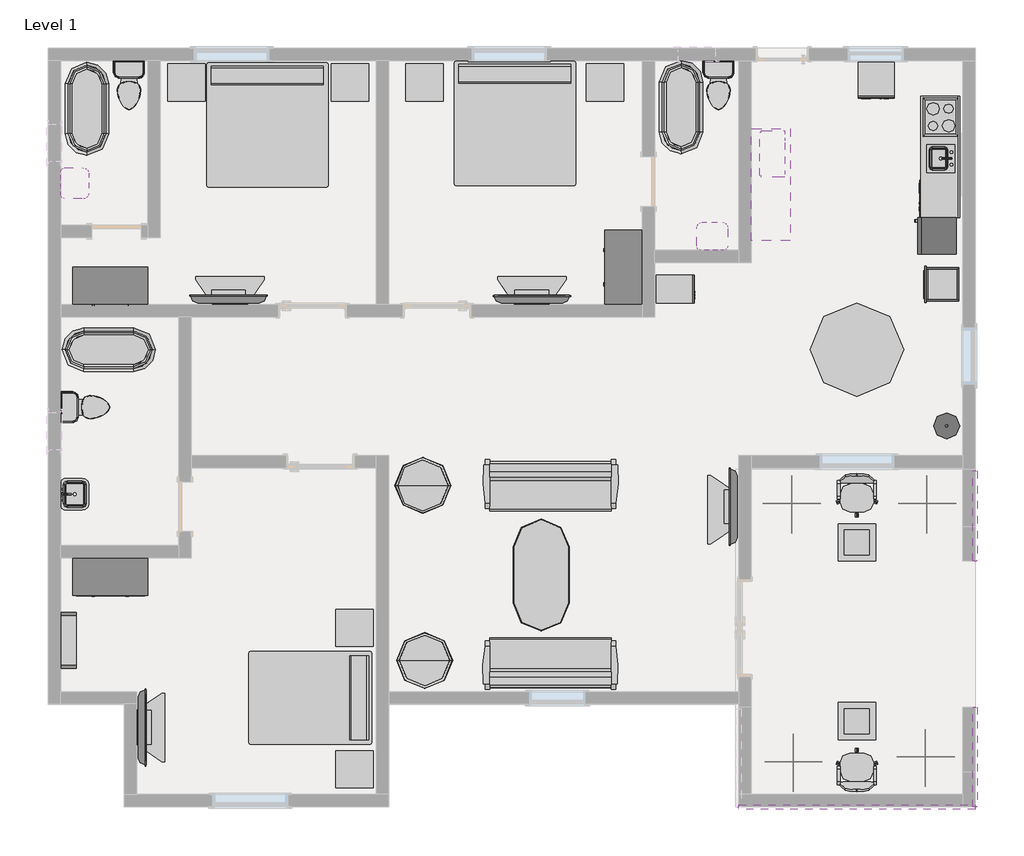
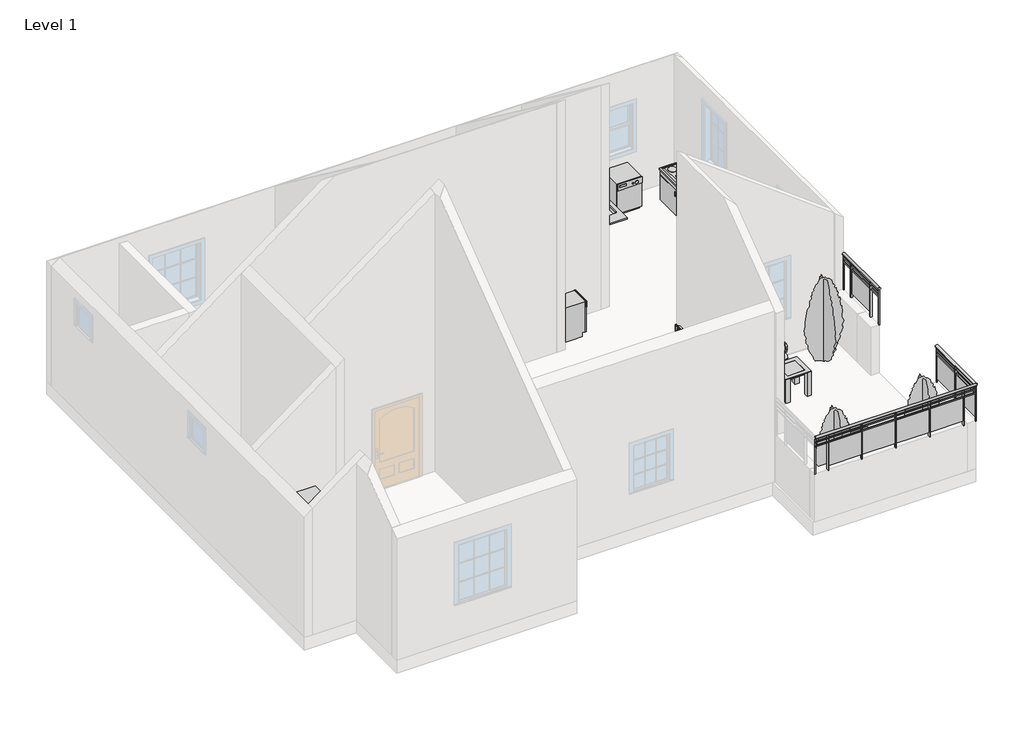
# One storey, part 2 of 2: 33 furniture elements, 11 flow terminals, 8 proxies, 4 geographic elements, 3 railings.
"""IFC4 building model written with IfcOpenShell, lengths in millimetres."""

from ifc_helpers import new_model, si_unit, point, frame, origin, place, context, project, spatial, polyline, ellipse_curve, trimmed, outline, extrude, transform, mapped, element, save
from ifc_brep_helpers import plane_surface, extruded_surface, advanced_brep
from components import proxy_7e1014cc, proxy_a6faaae8, proxy_53e5fb40, proxy_45b28599, kitchenette_medium_kitchenette_medium_844211aa, proxy_8a8d5ab2, proxy_8b8c2dc4, proxy_c523a7b7, flow_terminal_871c2e40, flow_terminal_d49f872f, flow_terminal_62a433f7, toilet_domestic_3d_toilet_domestic_3d_f7549cf7, toilet_domestic_3d_toilet_domestic_3d_183bbd19, flow_terminal_9fc66f1c, furniture_1fc5af50, furniture_e1791683, chair_executive_chair_executive_8d69e98c, furniture_c6510c7c, furniture_1447f48d, furniture_9fa109b2, furniture_417d203a, furniture_aff9b2fb, furniture_fdf74506, tv_stand_tv_stand_6ce107e5, furniture_b5c51a22, furniture_2c34a4f9, furniture_bbcc68ce, furniture_5bc9ed15, furniture_c80d6d9c, rpc_tree_conifer_chinese_juniper_7_1b9786cd

model = new_model("IFC4")

# Units and contexts
model_context = context("Model", 3, world=origin())
ifc_project = project(units=[si_unit("LENGTHUNIT", "METRE", prefix="MILLI")], contexts=[model_context])

# Site, building, storey
site = spatial("IfcSite", under=ifc_project)
building = spatial("IfcBuilding", under=site)
storey = spatial("IfcBuildingStorey", under=building, Name="Level 1", Elevation=0.0)

# Proxies
placement = place(None, origin())
proxy_shape = proxy_7e1014cc(model_context)
element("IfcBuildingElementProxy", 1, Name="18\" x 24\" x 34 1/2\"", ObjectType="18\" x 24\" x 34 1/2\"", at=placement, inside=storey, context=model_context, shape_type="MappedRepresentation", body=[
    mapped(proxy_shape, transform((-2808.5456342, 2713.390204, 0.0), x_axis=(0.0, 1.0000000000000002, 0.0), y_axis=(-1.0000000000000002, 0.0, 0.0), z_axis=(0.0, 0.0, 1.0))),
])
proxy_2_shape = proxy_a6faaae8(model_context)
element("IfcBuildingElementProxy", 2, Name="Cook Top-4 Unit2 : 22\" x 20\"", ObjectType="Cook Top-4 Unit2 : 22\" x 20\"", at=placement, inside=storey, context=model_context, shape_type="MappedRepresentation", body=[
    mapped(proxy_2_shape, transform((1268.404801, 5826.2076725, 0.0), x_axis=(0.0, -1.0, 0.0), y_axis=(1.0, 0.0, 0.0), z_axis=(0.0, 0.0, 1.0))),
])
proxy_3_shape = proxy_53e5fb40(model_context)
element("IfcBuildingElementProxy", 3, Name="Dishwasher : 23\" x 23 11/16\" x 33 1/2\"", ObjectType="Dishwasher : 23\" x 23 11/16\" x 33 1/2\"", at=placement, inside=storey, context=model_context, shape_type="MappedRepresentation", body=[
    mapped(proxy_3_shape, transform((-155.3126675, 6189.9956077, 0.0), x_axis=(1.0, 0.0, 0.0), y_axis=(0.0, 1.0, 0.0), z_axis=(0.0, 0.0, 1.0))),
])
proxy_4_shape = proxy_45b28599(model_context)
element("IfcBuildingElementProxy", 4, Name="Dishwasher : 24\" x 24\" x 34\"", ObjectType="Dishwasher : 24\" x 24\" x 34\"", at=placement, inside=storey, context=model_context, shape_type="MappedRepresentation", body=[
    mapped(proxy_4_shape, transform((976.5552362, 4875.025141, 0.0), x_axis=(0.0, -1.0, 0.0), y_axis=(1.0, 0.0, 0.0), z_axis=(0.0, 0.0, 1.0))),
])
kitchenette_medium_kitchenette_medium_shape = kitchenette_medium_kitchenette_medium_844211aa(model_context)
element("IfcBuildingElementProxy", 5, Name="Kitchenette - Medium : Kitchenette - Medium", ObjectType="Kitchenette - Medium : Kitchenette - Medium", at=placement, inside=storey, context=model_context, shape_type="MappedRepresentation", body=[
    mapped(kitchenette_medium_kitchenette_medium_shape, transform((1573.204801, 5502.0453774, 0.0), x_axis=(0.0, -1.0, 0.0), y_axis=(1.0, 0.0, 0.0), z_axis=(0.0, 0.0, 1.0))),
])
proxy_5_shape = proxy_8a8d5ab2(model_context)
element("IfcBuildingElementProxy", 6, Name="Microwave : 30\" x 16\" x 18\"", ObjectType="Microwave : 30\" x 16\" x 18\"", at=placement, inside=storey, context=model_context, shape_type="MappedRepresentation", body=[
    mapped(proxy_5_shape, transform((-1840.5757048, 4729.0147952, 914.4), x_axis=(0.0, 1.0000000000000002, 0.0), y_axis=(-1.0000000000000002, 0.0, 0.0), z_axis=(0.0, 0.0, 1.0))),
])
proxy_6_shape = proxy_8b8c2dc4(model_context)
element("IfcBuildingElementProxy", 7, Name="Oven Double-Built-in : 21 1/2\" x 39 1/4\" x 21\"", ObjectType="Oven Double-Built-in : 21 1/2\" x 39 1/4\" x 21\"", at=placement, inside=storey, context=model_context, shape_type="MappedRepresentation", body=[
    mapped(proxy_6_shape, transform((1152.7389421, 3060.5327452, 0.0), x_axis=(0.0, -1.0000000000000007, 0.0), y_axis=(1.0000000000000007, 0.0, 0.0), z_axis=(0.0, 0.0, 1.0))),
])
proxy_7_shape = proxy_c523a7b7(model_context)
element("IfcBuildingElementProxy", 8, Name="Refrigerator : 24\" x 25\" LH", ObjectType="Refrigerator : 24\" x 25\" LH", at=placement, inside=storey, context=model_context, shape_type="MappedRepresentation", body=[
    mapped(proxy_7_shape, transform((1222.7558295, 3889.4576725, 0.0), x_axis=(0.0, -1.0, 0.0), y_axis=(1.0, 0.0, 0.0), z_axis=(0.0, 0.0, 1.0))),
])

# Flow terminals
flow_terminal_shape = flow_terminal_871c2e40(model_context)
element("IfcFlowTerminal", 9, ObjectType="Sink Kitchen-Island : 18\" x 18\"", at=placement, inside=storey, context=model_context, shape_type="MappedRepresentation", body=[
    mapped(flow_terminal_shape, transform((1266.0593999, 5168.7969131, -14.4), x_axis=(0.0, -1.0, 0.0), y_axis=(1.0, 0.0, 0.0), z_axis=(0.0, 0.0, 1.0))),
])
flow_terminal_2_shape = flow_terminal_d49f872f(model_context)
element("IfcFlowTerminal", 10, ObjectType="Sink Vanity-Round : 19\" x 19\"", at=placement, inside=storey, context=model_context, shape_type="MappedRepresentation", body=[
    mapped(flow_terminal_2_shape, transform((1277.3399031, 880.9594131, 609.6), x_axis=(0.0, -1.0000000000000004, 0.0), y_axis=(1.0000000000000004, 0.0, 0.0), z_axis=(0.0, 0.0, 1.0))),
])
flow_terminal_3_shape = flow_terminal_62a433f7(model_context)
element("IfcFlowTerminal", 11, ObjectType="Sink Vanity-Square : 20\" x 18\"", at=placement, inside=storey, context=model_context, shape_type="MappedRepresentation", body=[
    mapped(flow_terminal_3_shape, transform((-12927.8497979, -348.9815681, 0.0), x_axis=(0.0, 1.0000000000000002, 0.0), y_axis=(-1.0000000000000002, 0.0, 0.0), z_axis=(0.0, 0.0, 1.0))),
])
element("IfcFlowTerminal", 12, ObjectType="Sink Vanity-Square : 20\" x 18\"", at=placement, inside=storey, context=model_context, shape_type="MappedRepresentation", body=[
    mapped(flow_terminal_3_shape, transform((-12927.8497979, 4731.0184319, 914.4), x_axis=(0.0, 1.0000000000000002, 0.0), y_axis=(-1.0000000000000002, 0.0, 0.0), z_axis=(0.0, 0.0, 1.0))),
])
element("IfcFlowTerminal", 13, ObjectType="Sink Vanity-Square : 20\" x 18\"", at=placement, inside=storey, context=model_context, shape_type="MappedRepresentation", body=[
    mapped(flow_terminal_3_shape, transform((-2449.7059584, 3834.6530736, 914.4), x_axis=(-1.0, 0.0, 0.0), y_axis=(0.0, -1.0, 0.0), z_axis=(0.0, 0.0, 1.0))),
])
toilet_domestic_3d_toilet_domestic_3d_shape = toilet_domestic_3d_toilet_domestic_3d_f7549cf7(model_context)
toilet_domestic_3d_toilet_domestic_3d_2_shape = toilet_domestic_3d_toilet_domestic_3d_183bbd19(model_context)
element("IfcFlowTerminal", 14, ObjectType="Toilet-Domestic-3D : Toilet-Domestic-3D", at=placement, inside=storey, context=model_context, shape_type="MappedRepresentation", body=[
    mapped(toilet_domestic_3d_toilet_domestic_3d_shape, transform((-12613.2991716, 1089.1076725, 0.0), x_axis=(0.0, 1.0000000000000002, 0.0), y_axis=(-1.0000000000000002, 0.0, 0.0), z_axis=(0.0, 0.0, 1.0))),
    mapped(toilet_domestic_3d_toilet_domestic_3d_2_shape, transform((-12613.2991716, 1089.1076725, 0.0), x_axis=(0.0, 1.0000000000000002, 0.0), y_axis=(-1.0000000000000002, 0.0, 0.0), z_axis=(0.0, 0.0, 1.0))),
])
element("IfcFlowTerminal", 15, ObjectType="Toilet-Domestic-3D : Toilet-Domestic-3D", at=placement, inside=storey, context=model_context, shape_type="MappedRepresentation", body=[
    mapped(toilet_domestic_3d_toilet_domestic_3d_shape, transform((-11990.395199, 6258.6116451, 0.0), x_axis=(1.0, 0.0, 0.0), y_axis=(0.0, 1.0, 0.0), z_axis=(0.0, 0.0, 1.0))),
    mapped(toilet_domestic_3d_toilet_domestic_3d_2_shape, transform((-11990.395199, 6258.6116451, 0.0), x_axis=(1.0, 0.0, 0.0), y_axis=(0.0, 1.0, 0.0), z_axis=(0.0, 0.0, 1.0))),
])
element("IfcFlowTerminal", 16, ObjectType="Toilet-Domestic-3D : Toilet-Domestic-3D", at=placement, inside=storey, context=model_context, shape_type="MappedRepresentation", body=[
    mapped(toilet_domestic_3d_toilet_domestic_3d_shape, transform((-2363.795199, 6258.6116451, 0.0), x_axis=(1.0, 0.0, 0.0), y_axis=(0.0, 1.0, 0.0), z_axis=(0.0, 0.0, 1.0))),
    mapped(toilet_domestic_3d_toilet_domestic_3d_2_shape, transform((-2363.795199, 6258.6116451, 0.0), x_axis=(1.0, 0.0, 0.0), y_axis=(0.0, 1.0, 0.0), z_axis=(0.0, 0.0, 1.0))),
])
flow_terminal_4_shape = flow_terminal_9fc66f1c(model_context)
element("IfcFlowTerminal", 17, ObjectType="Tub-Free Standing-3D : 30\" x 60\"", at=placement, inside=storey, context=model_context, shape_type="MappedRepresentation", body=[
    mapped(flow_terminal_4_shape, transform((-12320.595199, 2028.9076725, 0.0), x_axis=(0.0, 1.0000000000000009, 0.0), y_axis=(-1.0000000000000009, 0.0, 0.0), z_axis=(0.0, 0.0, 1.0))),
])
element("IfcFlowTerminal", 18, ObjectType="Tub-Free Standing-3D : 30\" x 60\"", at=placement, inside=storey, context=model_context, shape_type="MappedRepresentation", body=[
    mapped(flow_terminal_4_shape, transform((-12676.195199, 5965.9076725, 0.0), x_axis=(1.0, 0.0, 0.0), y_axis=(0.0, 1.0, 0.0), z_axis=(0.0, 0.0, 1.0))),
])
element("IfcFlowTerminal", 19, ObjectType="Tub-Free Standing-3D : 30\" x 60\"", at=placement, inside=storey, context=model_context, shape_type="MappedRepresentation", body=[
    mapped(flow_terminal_4_shape, transform((-2973.395199, 5991.3076725, 0.0), x_axis=(1.0, 0.0, 0.0), y_axis=(0.0, 1.0, 0.0), z_axis=(0.0, 0.0, 1.0))),
])

# Furniture
furniture_shape = furniture_1fc5af50(model_context)
element("IfcFurniture", 20, ObjectType="Bed-Standard.0001 : King 78\" x 80\"", at=placement, inside=storey, context=model_context, shape_type="MappedRepresentation", body=[
    mapped(furniture_shape, transform((-10001.2837236, 5744.8027545, 0.0), x_axis=(1.0, 0.0, 0.0), y_axis=(0.0, 1.0, 0.0), z_axis=(0.0, 0.0, 1.0))),
])
element("IfcFurniture", 21, ObjectType="Bed-Standard.0001 : King 78\" x 80\"", at=placement, inside=storey, context=model_context, shape_type="MappedRepresentation", body=[
    mapped(furniture_shape, transform((-5958.5510914, 5770.2027545, 0.0), x_axis=(1.0000000000000002, 0.0, 0.0), y_axis=(0.0, 1.0000000000000002, 0.0), z_axis=(0.0, 0.0, 1.0))),
])
furniture_2_shape = furniture_e1791683(model_context)
element("IfcFurniture", 22, ObjectType="Bed-Standard.0001 : Queen 60\" x 79\"", at=placement, inside=storey, context=model_context, shape_type="MappedRepresentation", body=[
    mapped(furniture_2_shape, transform((-8985.700117, -3389.2038029, 0.0), x_axis=(0.0, -1.0000000000000007, 0.0), y_axis=(1.0000000000000007, 0.0, 0.0), z_axis=(0.0, 0.0, 1.0))),
])
chair_executive_chair_executive_shape = chair_executive_chair_executive_8d69e98c(model_context)
element("IfcFurniture", 23, ObjectType="Chair-Executive : Chair-Executive", at=placement, inside=storey, context=model_context, shape_type="MappedRepresentation", body=[
    mapped(chair_executive_chair_executive_shape, transform((37.7956207, -339.7464259, 0.0), x_axis=(-1.0000000000000002, 0.0, 0.0), y_axis=(0.0, -1.0000000000000002, 0.0), z_axis=(0.0, 0.0, 1.0))),
])
element("IfcFurniture", 24, ObjectType="Chair-Executive : Chair-Executive", at=placement, inside=storey, context=model_context, shape_type="MappedRepresentation", body=[
    mapped(chair_executive_chair_executive_shape, transform((-244.1860187, -4848.0382291, 0.0), x_axis=(1.0000000000000002, 0.0, 0.0), y_axis=(0.0, 1.0000000000000002, 0.0), z_axis=(0.0, 0.0, 1.0))),
])
furniture_3_shape = furniture_c6510c7c(model_context)
element("IfcFurniture", 25, ObjectType="Counter Top w Sink Hole : 24\" Depth", at=placement, inside=storey, context=model_context, shape_type="MappedRepresentation", body=[
    mapped(furniture_3_shape, transform((1573.204801, 4968.6453774, -14.4), x_axis=(0.0, -1.0, 0.0), y_axis=(1.0, 0.0, 0.0), z_axis=(0.0, 0.0, 1.0))),
])
furniture_4_shape = furniture_1447f48d(model_context)
element("IfcFurniture", 26, ObjectType="Counter Top w Sink Hole : 24\" Depth", at=placement, inside=storey, context=model_context, shape_type="MappedRepresentation", body=[
    mapped(furniture_4_shape, transform((-1830.395199, 5007.3699676, 914.4), x_axis=(0.0, 1.0000000000000002, 0.0), y_axis=(-1.0000000000000002, 0.0, 0.0), z_axis=(0.0, 0.0, 1.0))),
])
furniture_5_shape = furniture_9fa109b2(model_context)
element("IfcFurniture", 27, ObjectType="Dresser : 48\" x 72\" x 24\"", at=placement, inside=storey, context=model_context, shape_type="MappedRepresentation", body=[
    mapped(furniture_5_shape, transform((-12026.0019391, 3433.4706266, 0.0), x_axis=(1.0, 0.0, 0.0), y_axis=(0.0, 1.0, 0.0), z_axis=(0.0, 0.0, 1.0))),
])
element("IfcFurniture", 28, ObjectType="Dresser : 48\" x 72\" x 24\"", at=placement, inside=storey, context=model_context, shape_type="MappedRepresentation", body=[
    mapped(furniture_5_shape, transform((-12026.0019391, -1316.3293734, 0.0), x_axis=(1.0, 0.0, 0.0), y_axis=(0.0, 1.0, 0.0), z_axis=(0.0, 0.0, 1.0))),
])
element("IfcFurniture", 29, ObjectType="Dresser : 48\" x 72\" x 24\"", at=placement, inside=storey, context=model_context, shape_type="MappedRepresentation", body=[
    mapped(furniture_5_shape, transform((-3550.0322449, 3105.9144127, 0.0), x_axis=(0.0, -1.0000000000000004, 0.0), y_axis=(1.0000000000000004, 0.0, 0.0), z_axis=(0.0, 0.0, 1.0))),
])
furniture_6_shape = furniture_417d203a(model_context)
element("IfcFurniture", 30, ObjectType="Shelving : 36\" x 10\" x 72\"", at=placement, inside=storey, context=model_context, shape_type="MappedRepresentation", body=[
    mapped(furniture_6_shape, transform((-13285.795199, -2720.8923275, 0.0), x_axis=(0.0, 1.0, 0.0), y_axis=(-1.0, 0.0, 0.0), z_axis=(0.0, 0.0, 1.0))),
])
furniture_7_shape = furniture_aff9b2fb(model_context)
element("IfcFurniture", 31, ObjectType="Sofa-Pensi : 84\"", at=placement, inside=storey, context=model_context, shape_type="MappedRepresentation", body=[
    mapped(furniture_7_shape, transform((-5385.601449, -464.3521636, 0.0), x_axis=(1.0000000000000009, 0.0, 0.0), y_axis=(0.0, 1.0000000000000009, 0.0), z_axis=(0.0, 0.0, 1.0))),
])
element("IfcFurniture", 32, ObjectType="Sofa-Pensi : 84\"", at=placement, inside=storey, context=model_context, shape_type="MappedRepresentation", body=[
    mapped(furniture_7_shape, transform((-4828.388949, -2824.7824914, 0.0), x_axis=(-1.0, 0.0, 0.0), y_axis=(0.0, -1.0, 0.0), z_axis=(0.0, 0.0, 1.0))),
])
furniture_8_shape = furniture_fdf74506(model_context)
element("IfcFurniture", 33, ObjectType="TV - Flat Screen : 50\"", at=placement, inside=storey, context=model_context, shape_type="MappedRepresentation", body=[
    mapped(furniture_8_shape, transform((-10368.7397131, 2850.4920708, 914.4), x_axis=(-1.0, 0.0, 0.0), y_axis=(0.0, -1.0, 0.0), z_axis=(0.0, 0.0, 1.0))),
])
element("IfcFurniture", 34, ObjectType="TV - Flat Screen : 50\"", at=placement, inside=storey, context=model_context, shape_type="MappedRepresentation", body=[
    mapped(furniture_8_shape, transform((-5415.7397131, 2847.8196508, 914.4), x_axis=(-1.0, 0.0, 0.0), y_axis=(0.0, -1.0, 0.0), z_axis=(0.0, 0.0, 1.0))),
])
element("IfcFurniture", 35, ObjectType="TV - Flat Screen : 50\"", at=placement, inside=storey, context=model_context, shape_type="MappedRepresentation", body=[
    mapped(furniture_8_shape, transform((-11779.4565753, -4139.3478134, 914.4), x_axis=(0.0, 1.0000000000000002, 0.0), y_axis=(-1.0000000000000002, 0.0, 0.0), z_axis=(0.0, 0.0, 1.0))),
])
element("IfcFurniture", 36, ObjectType="TV - Flat Screen : 50\"", at=placement, inside=storey, context=model_context, shape_type="MappedRepresentation", body=[
    mapped(furniture_8_shape, transform((-2117.5338226, -540.4368416, 914.4), x_axis=(0.0, -1.0000000000000002, 0.0), y_axis=(1.0000000000000002, 0.0, 0.0), z_axis=(0.0, 0.0, 1.0))),
])
tv_stand_tv_stand_shape = tv_stand_tv_stand_6ce107e5(model_context)
element("IfcFurniture", 37, ObjectType="TV Stand : TV Stand", at=placement, inside=storey, context=model_context, shape_type="MappedRepresentation", body=[
    mapped(tv_stand_tv_stand_shape, transform((-11863.395199, -4268.4803296, 0.0), x_axis=(0.0, 1.0, 0.0), y_axis=(-1.0, 0.0, 0.0), z_axis=(0.0, 0.0, 1.0))),
])
element("IfcFurniture", 38, ObjectType="TV Stand : TV Stand", at=placement, inside=storey, context=model_context, shape_type="MappedRepresentation", body=[
    mapped(tv_stand_tv_stand_shape, transform((-10214.2071969, 2765.5076725, 0.0), x_axis=(-1.0000000000000002, 0.0, 0.0), y_axis=(0.0, -1.0000000000000002, 0.0), z_axis=(0.0, 0.0, 1.0))),
])
element("IfcFurniture", 39, ObjectType="TV Stand : TV Stand", at=placement, inside=storey, context=model_context, shape_type="MappedRepresentation", body=[
    mapped(tv_stand_tv_stand_shape, transform((-5286.6071969, 2765.5076725, 0.0), x_axis=(-1.0, 0.0, 0.0), y_axis=(0.0, -1.0, 0.0), z_axis=(0.0, 0.0, 1.0))),
])
element("IfcFurniture", 40, ObjectType="TV Stand : TV Stand", at=placement, inside=storey, context=model_context, shape_type="MappedRepresentation", body=[
    mapped(tv_stand_tv_stand_shape, transform((-2084.395199, -462.1043254, 0.0), x_axis=(0.0, -1.0, 0.0), y_axis=(1.0, 0.0, 0.0), z_axis=(0.0, 0.0, 1.0))),
])
furniture_9_shape = furniture_b5c51a22(model_context)
element("IfcFurniture", 41, ObjectType="Table-Coffee : 24\" x 24\" x 24\"", at=placement, inside=storey, context=model_context, shape_type="MappedRepresentation", body=[
    mapped(furniture_9_shape, transform((-121.4609657, -4136.9034053, 0.0), x_axis=(1.0, 0.0, 0.0), y_axis=(0.0, 1.0, 0.0), z_axis=(0.0, 0.0, 1.0))),
])
element("IfcFurniture", 42, ObjectType="Table-Coffee : 24\" x 24\" x 24\"", at=placement, inside=storey, context=model_context, shape_type="MappedRepresentation", body=[
    mapped(furniture_9_shape, transform((-121.4609657, -1215.9034053, 0.0), x_axis=(1.0, 0.0, 0.0), y_axis=(0.0, 1.0, 0.0), z_axis=(0.0, 0.0, 1.0))),
])
furniture_10_shape = furniture_2c34a4f9(model_context)
element("IfcFurniture", 43, ObjectType="Table-Dining Oval : 36\" x 72\"", at=placement, inside=storey, context=model_context, shape_type="MappedRepresentation", body=[
    mapped(furniture_10_shape, transform((-5617.4935596, -1252.2726554, 0.0), x_axis=(0.0, 1.0000000000000002, 0.0), y_axis=(-1.0000000000000002, 0.0, 0.0), z_axis=(0.0, 0.0, 1.0))),
])
furniture_11_shape = furniture_bbcc68ce(model_context)
element("IfcFurniture", 44, ObjectType="Table-Dining Round w Chairs : 60\" Diameter", at=placement, inside=storey, context=model_context, shape_type="MappedRepresentation", body=[
    mapped(furniture_11_shape, transform((-206.8771662, 2213.786361, 0.0), x_axis=(1.0, 0.0, 0.0), y_axis=(0.0, 1.0, 0.0), z_axis=(0.0, 0.0, 1.0))),
])
furniture_12_shape = furniture_5bc9ed15(model_context)
element("IfcFurniture", 45, ObjectType="Table-Night Stand : 24\" x 24\" x 30\"", at=placement, inside=storey, context=model_context, shape_type="MappedRepresentation", body=[
    mapped(furniture_12_shape, transform((-8692.1288293, 6092.9076725, 0.0), x_axis=(1.0, 0.0, 0.0), y_axis=(0.0, 1.0, 0.0), z_axis=(0.0, 0.0, 1.0))),
])
element("IfcFurniture", 46, ObjectType="Table-Night Stand : 24\" x 24\" x 30\"", at=placement, inside=storey, context=model_context, shape_type="MappedRepresentation", body=[
    mapped(furniture_12_shape, transform((-11359.1288293, 6092.9076725, 0.0), x_axis=(1.0, 0.0, 0.0), y_axis=(0.0, 1.0, 0.0), z_axis=(0.0, 0.0, 1.0))),
])
element("IfcFurniture", 47, ObjectType="Table-Night Stand : 24\" x 24\" x 30\"", at=placement, inside=storey, context=model_context, shape_type="MappedRepresentation", body=[
    mapped(furniture_12_shape, transform((-7472.9288293, 6092.9076725, 0.0), x_axis=(1.0, 0.0, 0.0), y_axis=(0.0, 1.0, 0.0), z_axis=(0.0, 0.0, 1.0))),
])
element("IfcFurniture", 48, ObjectType="Table-Night Stand : 24\" x 24\" x 30\"", at=placement, inside=storey, context=model_context, shape_type="MappedRepresentation", body=[
    mapped(furniture_12_shape, transform((-4526.5288293, 6092.9076725, 0.0), x_axis=(1.0, 0.0, 0.0), y_axis=(0.0, 1.0, 0.0), z_axis=(0.0, 0.0, 1.0))),
])
element("IfcFurniture", 49, ObjectType="Table-Night Stand : 24\" x 24\" x 30\"", at=placement, inside=storey, context=model_context, shape_type="MappedRepresentation", body=[
    mapped(furniture_12_shape, transform((-8615.9288293, -2822.4923275, 0.0), x_axis=(1.0, 0.0, 0.0), y_axis=(0.0, 1.0, 0.0), z_axis=(0.0, 0.0, 1.0))),
])
element("IfcFurniture", 50, ObjectType="Table-Night Stand : 24\" x 24\" x 30\"", at=placement, inside=storey, context=model_context, shape_type="MappedRepresentation", body=[
    mapped(furniture_12_shape, transform((-8615.9288293, -5133.8923275, 0.0), x_axis=(1.0, 0.0, 0.0), y_axis=(0.0, 1.0, 0.0), z_axis=(0.0, 0.0, 1.0))),
])
furniture_13_shape = furniture_c80d6d9c(model_context)
element("IfcFurniture", 51, ObjectType="Table-Round : 36\" Diameter", at=placement, inside=storey, context=model_context, shape_type="MappedRepresentation", body=[
    mapped(furniture_13_shape, transform((-7164.395199, -3051.0923275, 0.0), x_axis=(1.0, 0.0, 0.0), y_axis=(0.0, 1.0, 0.0), z_axis=(0.0, 0.0, 1.0))),
])
element("IfcFurniture", 52, ObjectType="Table-Round : 36\" Diameter", at=placement, inside=storey, context=model_context, shape_type="MappedRepresentation", body=[
    mapped(furniture_13_shape, transform((-7189.795199, -187.2423275, 0.0), x_axis=(1.0, 0.0, 0.0), y_axis=(0.0, 1.0, 0.0), z_axis=(0.0, 0.0, 1.0))),
])

# Geographic elements
rpc_tree_conifer_chinese_juniper_7_shape = rpc_tree_conifer_chinese_juniper_7_1b9786cd(model_context)
element("IfcGeographicElement", 53, ObjectType="RPC Tree - Conifer : Chinese Juniper - 7'", at=placement, inside=storey, context=model_context, shape_type="MappedRepresentation", body=[
    mapped(rpc_tree_conifer_chinese_juniper_7_shape, transform((-1144.7918701, -4702.0923275, 0.0), x_axis=(1.0, 0.0, 0.0), y_axis=(0.0, 1.0, 0.0), z_axis=(0.0, 0.0, 1.0))),
])
element("IfcGeographicElement", 54, ObjectType="RPC Tree - Conifer : Chinese Juniper - 7'", at=placement, inside=storey, context=model_context, shape_type="MappedRepresentation", body=[
    mapped(rpc_tree_conifer_chinese_juniper_7_shape, transform((1014.2081299, -4625.8923275, 0.0), x_axis=(1.0, 0.0, 0.0), y_axis=(0.0, 1.0, 0.0), z_axis=(0.0, 0.0, 1.0))),
])
element("IfcGeographicElement", 55, ObjectType="RPC Tree - Conifer : Chinese Juniper - 7'", at=placement, inside=storey, context=model_context, shape_type="MappedRepresentation", body=[
    mapped(rpc_tree_conifer_chinese_juniper_7_shape, transform((1039.6081299, -485.6923275, 0.0), x_axis=(1.0, 0.0, 0.0), y_axis=(0.0, 1.0, 0.0), z_axis=(0.0, 0.0, 1.0))),
])
element("IfcGeographicElement", 56, ObjectType="RPC Tree - Conifer : Chinese Juniper - 7'", at=placement, inside=storey, context=model_context, shape_type="MappedRepresentation", body=[
    mapped(rpc_tree_conifer_chinese_juniper_7_shape, transform((-1170.1918701, -485.6923275, 0.0), x_axis=(1.0, 0.0, 0.0), y_axis=(0.0, 1.0, 0.0), z_axis=(0.0, 0.0, 1.0))),
])

# Railings
element("IfcRailing", 57, ObjectType="Glass Panel - Bottom Fill", at=placement, inside=storey, context=model_context, shape_type="SolidModel", body=[
    advanced_brep(
    [(-2033.595199, -5406.9423275, 2133.6), (-2033.595199, -5483.1423275, 2133.6), (1827.204801, -5406.9423275, 2133.6), (1827.204801, -5483.1423275, 2133.6)],
    [
        (0, 1, ellipse_curve(frame((-2033.595199, -5445.0423275, 2133.6), z_axis=(-1.0, 0.0, 0.0), x_axis=(0.0, -1.0, 0.0)), 38.1, 28.575)),
        (1, 0, ellipse_curve(frame((-2033.595199, -5445.0423275, 2133.6), z_axis=(-1.0, 0.0, 0.0), x_axis=(0.0, -1.0, 0.0)), 38.1, 28.575)),
        (2, 3, ellipse_curve(frame((1827.204801, -5445.0423275, 2133.6), z_axis=(1.0, 0.0, 0.0), x_axis=(0.0, -1.0, 0.0)), 38.1, 28.575)),
        (3, 2, ellipse_curve(frame((1827.204801, -5445.0423275, 2133.6), z_axis=(1.0, 0.0, 0.0), x_axis=(0.0, -1.0, 0.0)), 38.1, 28.575)),
        (0, 2),
        (3, 1),
    ],
    [
        plane_surface(frame((-2033.595199, -5445.0423275, 2133.6), z_axis=(-1.0, 0.0, 0.0), x_axis=(0.0, 1.0, 0.0))),
        plane_surface(frame((1827.204801, -5445.0423275, 2133.6), z_axis=(1.0, 0.0, 0.0), x_axis=(0.0, 1.0, 0.0))),
        extruded_surface(trimmed(ellipse_curve(frame((1827.204801, -5445.0423275, 2133.6), z_axis=(-1.0, 0.0, 0.0), x_axis=(0.0, -1.0, 0.0)), 38.1, 28.575), [point((1827.204801, -5406.9423275, 2133.6))], [point((1827.204801, -5483.1423275, 2133.6))], True, "CARTESIAN"), (-3860.8, 0.0, 0.0), 3860.8),
        extruded_surface(trimmed(ellipse_curve(frame((1827.204801, -5445.0423275, 2133.6), z_axis=(-1.0, 0.0, 0.0), x_axis=(0.0, -1.0, 0.0)), 38.1, 28.575), [point((1827.204801, -5483.1423275, 2133.6))], [point((1827.204801, -5406.9423275, 2133.6))], True, "CARTESIAN"), (-3860.8, 0.0, 0.0), 3860.8),
    ],
    [
        (0, [[1, 2]]),
        (1, [[3, 4]]),
        (2, [[-1, 5, -4, 6]]),
        (3, [[-2, -6, -3, -5]]),
    ],
),
    extrude(outline(polyline([(-2033.595199, -5457.7423275), (-2033.595199, -5432.3423275), (1827.204801, -5432.3423275), (1827.204801, -5457.7423275), (-2033.595199, -5457.7423275)])), frame((0.0, 0.0, 2019.3), z_axis=(0.0, 0.0, 1.0), x_axis=(1.0, 0.0, 0.0)), (0.0, 0.0, 1.0), 25.4),
    extrude(outline(polyline([(-2033.595199, -5457.7423275), (-2033.595199, -5432.3423275), (1827.204801, -5432.3423275), (1827.204801, -5457.7423275), (-2033.595199, -5457.7423275)])), frame((0.0, 0.0, 1917.7), z_axis=(0.0, 0.0, 1.0), x_axis=(1.0, 0.0, 0.0)), (0.0, 0.0, 1.0), 25.4),
    extrude(outline(polyline([(1516.054801, -5470.4423275), (1516.054801, -5419.6423275), (1528.754801, -5419.6423275), (1528.754801, -5470.4423275), (1516.054801, -5470.4423275)])), frame((0.0, 0.0, 1219.2), z_axis=(0.0, 0.0, 1.0), x_axis=(1.0, 0.0, 0.0)), (0.0, 0.0, 1.0), 885.6788223),
    extrude(outline(polyline([(709.604801, -5438.5071705), (1522.404801, -5438.5071705), (1522.404801, -5444.8571705), (709.604801, -5444.8571705), (709.604801, -5438.5071705)])), frame((0.0, 0.0, 1320.8), z_axis=(0.0, 0.0, 1.0), x_axis=(1.0, 0.0, 0.0)), (0.0, 0.0, 1.0), 596.9),
    extrude(outline(polyline([(703.254801, -5470.4423275), (703.254801, -5419.6423275), (715.954801, -5419.6423275), (715.954801, -5470.4423275), (703.254801, -5470.4423275)])), frame((0.0, 0.0, 1219.2), z_axis=(0.0, 0.0, 1.0), x_axis=(1.0, 0.0, 0.0)), (0.0, 0.0, 1.0), 885.6788223),
    extrude(outline(polyline([(-103.195199, -5438.5071705), (709.604801, -5438.5071705), (709.604801, -5444.8571705), (-103.195199, -5444.8571705), (-103.195199, -5438.5071705)])), frame((0.0, 0.0, 1320.8), z_axis=(0.0, 0.0, 1.0), x_axis=(1.0, 0.0, 0.0)), (0.0, 0.0, 1.0), 596.9),
    extrude(outline(polyline([(-109.545199, -5470.4423275), (-109.545199, -5419.6423275), (-96.845199, -5419.6423275), (-96.845199, -5470.4423275), (-109.545199, -5470.4423275)])), frame((0.0, 0.0, 1219.2), z_axis=(0.0, 0.0, 1.0), x_axis=(1.0, 0.0, 0.0)), (0.0, 0.0, 1.0), 885.6788223),
    extrude(outline(polyline([(-915.995199, -5438.5071705), (-103.195199, -5438.5071705), (-103.195199, -5444.8571705), (-915.995199, -5444.8571705), (-915.995199, -5438.5071705)])), frame((0.0, 0.0, 1320.8), z_axis=(0.0, 0.0, 1.0), x_axis=(1.0, 0.0, 0.0)), (0.0, 0.0, 1.0), 596.9),
    extrude(outline(polyline([(-922.345199, -5470.4423275), (-922.345199, -5419.6423275), (-909.645199, -5419.6423275), (-909.645199, -5470.4423275), (-922.345199, -5470.4423275)])), frame((0.0, 0.0, 1219.2), z_axis=(0.0, 0.0, 1.0), x_axis=(1.0, 0.0, 0.0)), (0.0, 0.0, 1.0), 885.6788223),
    extrude(outline(polyline([(-1728.795199, -5438.5071705), (-915.995199, -5438.5071705), (-915.995199, -5444.8571705), (-1728.795199, -5444.8571705), (-1728.795199, -5438.5071705)])), frame((0.0, 0.0, 1320.8), z_axis=(0.0, 0.0, 1.0), x_axis=(1.0, 0.0, 0.0)), (0.0, 0.0, 1.0), 596.9),
    extrude(outline(polyline([(-1735.145199, -5470.4423275), (-1735.145199, -5419.6423275), (-1722.445199, -5419.6423275), (-1722.445199, -5470.4423275), (-1735.145199, -5470.4423275)])), frame((0.0, 0.0, 1219.2), z_axis=(0.0, 0.0, 1.0), x_axis=(1.0, 0.0, 0.0)), (0.0, 0.0, 1.0), 885.6788223),
    extrude(outline(polyline([(1814.504801, -5454.5673275), (1814.504801, -5435.5173275), (1833.554801, -5435.5173275), (1833.554801, -5454.5673275), (1814.504801, -5454.5673275)])), frame((0.0, 0.0, 1219.2), z_axis=(0.0, 0.0, 1.0), x_axis=(1.0, 0.0, 0.0)), (0.0, 0.0, 1.0), 885.6788223),
    extrude(outline(polyline([(-2039.945199, -5454.5673275), (-2039.945199, -5435.5173275), (-2020.895199, -5435.5173275), (-2020.895199, -5454.5673275), (-2039.945199, -5454.5673275)])), frame((0.0, 0.0, 1219.2), z_axis=(0.0, 0.0, 1.0), x_axis=(1.0, 0.0, 0.0)), (0.0, 0.0, 1.0), 885.6788223),
])
element("IfcRailing", 58, ObjectType="Glass Panel - Bottom Fill", at=placement, inside=storey, context=model_context, shape_type="SolidModel", body=[
    advanced_brep(
    [(1789.104801, -5438.6923275, 2133.6), (1865.304801, -5438.6923275, 2133.6), (1789.104801, -3813.0923275, 2133.6), (1865.304801, -3813.0923275, 2133.6)],
    [
        (0, 1, ellipse_curve(frame((1827.204801, -5438.6923275, 2133.6), z_axis=(0.0, -1.0, 0.0), x_axis=(1.0, 0.0, 0.0)), 38.1, 28.575)),
        (1, 0, ellipse_curve(frame((1827.204801, -5438.6923275, 2133.6), z_axis=(0.0, -1.0, 0.0), x_axis=(1.0, 0.0, 0.0)), 38.1, 28.575)),
        (2, 3, ellipse_curve(frame((1827.204801, -3813.0923275, 2133.6), z_axis=(0.0, 1.0, 0.0), x_axis=(1.0, 0.0, 0.0)), 38.1, 28.575)),
        (3, 2, ellipse_curve(frame((1827.204801, -3813.0923275, 2133.6), z_axis=(0.0, 1.0, 0.0), x_axis=(1.0, 0.0, 0.0)), 38.1, 28.575)),
        (0, 2),
        (3, 1),
    ],
    [
        plane_surface(frame((1827.204801, -5438.6923275, 2133.6), z_axis=(0.0, -1.0, 0.0), x_axis=(0.0, 0.0, 1.0))),
        plane_surface(frame((1827.204801, -3813.0923275, 2133.6), z_axis=(0.0, 1.0, 0.0), x_axis=(0.0, 0.0, 1.0))),
        extruded_surface(trimmed(ellipse_curve(frame((1827.204801, -3813.0923275, 2133.6), z_axis=(0.0, -1.0, 0.0), x_axis=(1.0, 0.0, 0.0)), 38.1, 28.575), [point((1789.104801, -3813.0923275, 2133.6))], [point((1865.304801, -3813.0923275, 2133.6))], True, "CARTESIAN"), (0.0, -1625.6, 0.0), 1625.6),
        extruded_surface(trimmed(ellipse_curve(frame((1827.204801, -3813.0923275, 2133.6), z_axis=(0.0, -1.0, 0.0), x_axis=(1.0, 0.0, 0.0)), 38.1, 28.575), [point((1865.304801, -3813.0923275, 2133.6))], [point((1789.104801, -3813.0923275, 2133.6))], True, "CARTESIAN"), (0.0, -1625.6, 0.0), 1625.6),
    ],
    [
        (0, [[1, 2]]),
        (1, [[3, 4]]),
        (2, [[-1, 5, -4, 6]]),
        (3, [[-2, -6, -3, -5]]),
    ],
),
    extrude(outline(polyline([(1839.904801, -5438.6923275), (1814.504801, -5438.6923275), (1814.504801, -3813.0923275), (1839.904801, -3813.0923275), (1839.904801, -5438.6923275)])), frame((0.0, 0.0, 2019.3), z_axis=(0.0, 0.0, 1.0), x_axis=(1.0, 0.0, 0.0)), (0.0, 0.0, 1.0), 25.4),
    extrude(outline(polyline([(1839.904801, -5438.6923275), (1814.504801, -5438.6923275), (1814.504801, -3813.0923275), (1839.904801, -3813.0923275), (1839.904801, -5438.6923275)])), frame((0.0, 0.0, 1917.7), z_axis=(0.0, 0.0, 1.0), x_axis=(1.0, 0.0, 0.0)), (0.0, 0.0, 1.0), 25.4),
    extrude(outline(polyline([(1820.669644, -4625.8923275), (1820.669644, -3813.0923275), (1827.019644, -3813.0923275), (1827.019644, -4625.8923275), (1820.669644, -4625.8923275)])), frame((0.0, 0.0, 1320.8), z_axis=(0.0, 0.0, 1.0), x_axis=(1.0, 0.0, 0.0)), (0.0, 0.0, 1.0), 596.9),
    extrude(outline(polyline([(1852.604801, -4632.2423275), (1801.804801, -4632.2423275), (1801.804801, -4619.5423275), (1852.604801, -4619.5423275), (1852.604801, -4632.2423275)])), frame((0.0, 0.0, 1219.2), z_axis=(0.0, 0.0, 1.0), x_axis=(1.0, 0.0, 0.0)), (0.0, 0.0, 1.0), 885.6788223),
    extrude(outline(polyline([(1820.669644, -5438.6923275), (1820.669644, -4625.8923275), (1827.019644, -4625.8923275), (1827.019644, -5438.6923275), (1820.669644, -5438.6923275)])), frame((0.0, 0.0, 1320.8), z_axis=(0.0, 0.0, 1.0), x_axis=(1.0, 0.0, 0.0)), (0.0, 0.0, 1.0), 596.9),
    extrude(outline(polyline([(1836.729801, -3825.7923275), (1817.679801, -3825.7923275), (1817.679801, -3806.7423275), (1836.729801, -3806.7423275), (1836.729801, -3825.7923275)])), frame((0.0, 0.0, 1219.2), z_axis=(0.0, 0.0, 1.0), x_axis=(1.0, 0.0, 0.0)), (0.0, 0.0, 1.0), 885.6788223),
    extrude(outline(polyline([(1836.729801, -5445.0423275), (1817.679801, -5445.0423275), (1817.679801, -5425.9923275), (1836.729801, -5425.9923275), (1836.729801, -5445.0423275)])), frame((0.0, 0.0, 1219.2), z_axis=(0.0, 0.0, 1.0), x_axis=(1.0, 0.0, 0.0)), (0.0, 0.0, 1.0), 885.6788223),
])
element("IfcRailing", 59, ObjectType="Glass Panel - Bottom Fill", at=placement, inside=storey, context=model_context, shape_type="SolidModel", body=[
    advanced_brep(
    [(1865.304801, 47.7076725, 2133.6), (1789.104801, 47.7076725, 2133.6), (1865.304801, -1425.4923275, 2133.6), (1789.104801, -1425.4923275, 2133.6)],
    [
        (0, 1, ellipse_curve(frame((1827.204801, 47.7076725, 2133.6), z_axis=(0.0, 1.0, 0.0), x_axis=(-1.0, 0.0, 0.0)), 38.1, 28.575)),
        (1, 0, ellipse_curve(frame((1827.204801, 47.7076725, 2133.6), z_axis=(0.0, 1.0, 0.0), x_axis=(-1.0, 0.0, 0.0)), 38.1, 28.575)),
        (2, 3, ellipse_curve(frame((1827.204801, -1425.4923275, 2133.6), z_axis=(0.0, -1.0, 0.0), x_axis=(-1.0, 0.0, 0.0)), 38.1, 28.575)),
        (3, 2, ellipse_curve(frame((1827.204801, -1425.4923275, 2133.6), z_axis=(0.0, -1.0, 0.0), x_axis=(-1.0, 0.0, 0.0)), 38.1, 28.575)),
        (0, 2),
        (3, 1),
    ],
    [
        plane_surface(frame((1827.204801, 47.7076725, 2133.6), z_axis=(0.0, 1.0, 0.0), x_axis=(0.0, 0.0, -1.0))),
        plane_surface(frame((1827.204801, -1425.4923275, 2133.6), z_axis=(0.0, -1.0, 0.0), x_axis=(0.0, 0.0, -1.0))),
        extruded_surface(trimmed(ellipse_curve(frame((1827.204801, -1425.4923275, 2133.6), z_axis=(0.0, 1.0, 0.0), x_axis=(-1.0, 0.0, 0.0)), 38.1, 28.575), [point((1865.304801, -1425.4923275, 2133.6))], [point((1789.104801, -1425.4923275, 2133.6))], True, "CARTESIAN"), (0.0, 1473.2, 0.0), 1473.2),
        extruded_surface(trimmed(ellipse_curve(frame((1827.204801, -1425.4923275, 2133.6), z_axis=(0.0, 1.0, 0.0), x_axis=(-1.0, 0.0, 0.0)), 38.1, 28.575), [point((1789.104801, -1425.4923275, 2133.6))], [point((1865.304801, -1425.4923275, 2133.6))], True, "CARTESIAN"), (0.0, 1473.2, 0.0), 1473.2),
    ],
    [
        (0, [[1, 2]]),
        (1, [[3, 4]]),
        (2, [[-1, 5, -4, 6]]),
        (3, [[-2, -6, -3, -5]]),
    ],
),
    extrude(outline(polyline([(1814.504801, 47.7076725), (1839.904801, 47.7076725), (1839.904801, -1425.4923275), (1814.504801, -1425.4923275), (1814.504801, 47.7076725)])), frame((0.0, 0.0, 2019.3), z_axis=(0.0, 0.0, 1.0), x_axis=(1.0, 0.0, 0.0)), (0.0, 0.0, 1.0), 25.4),
    extrude(outline(polyline([(1814.504801, 47.7076725), (1839.904801, 47.7076725), (1839.904801, -1425.4923275), (1814.504801, -1425.4923275), (1814.504801, 47.7076725)])), frame((0.0, 0.0, 1917.7), z_axis=(0.0, 0.0, 1.0), x_axis=(1.0, 0.0, 0.0)), (0.0, 0.0, 1.0), 25.4),
    extrude(outline(polyline([(1801.804801, -1088.9423275), (1852.604801, -1088.9423275), (1852.604801, -1101.6423275), (1801.804801, -1101.6423275), (1801.804801, -1088.9423275)])), frame((0.0, 0.0, 1219.2), z_axis=(0.0, 0.0, 1.0), x_axis=(1.0, 0.0, 0.0)), (0.0, 0.0, 1.0), 885.6788223),
    extrude(outline(polyline([(1833.739958, -282.4923275), (1833.739958, -1095.2923275), (1827.389958, -1095.2923275), (1827.389958, -282.4923275), (1833.739958, -282.4923275)])), frame((0.0, 0.0, 1320.8), z_axis=(0.0, 0.0, 1.0), x_axis=(1.0, 0.0, 0.0)), (0.0, 0.0, 1.0), 596.9),
    extrude(outline(polyline([(1801.804801, -276.1423275), (1852.604801, -276.1423275), (1852.604801, -288.8423275), (1801.804801, -288.8423275), (1801.804801, -276.1423275)])), frame((0.0, 0.0, 1219.2), z_axis=(0.0, 0.0, 1.0), x_axis=(1.0, 0.0, 0.0)), (0.0, 0.0, 1.0), 885.6788223),
    extrude(outline(polyline([(1817.679801, -1412.7923275), (1836.729801, -1412.7923275), (1836.729801, -1431.8423275), (1817.679801, -1431.8423275), (1817.679801, -1412.7923275)])), frame((0.0, 0.0, 1219.2), z_axis=(0.0, 0.0, 1.0), x_axis=(1.0, 0.0, 0.0)), (0.0, 0.0, 1.0), 885.6788223),
    extrude(outline(polyline([(1817.679801, 54.0576725), (1836.729801, 54.0576725), (1836.729801, 35.0076725), (1817.679801, 35.0076725), (1817.679801, 54.0576725)])), frame((0.0, 0.0, 1219.2), z_axis=(0.0, 0.0, 1.0), x_axis=(1.0, 0.0, 0.0)), (0.0, 0.0, 1.0), 885.6788223),
])

save(model, "model.ifc")

# Revit data of these elements
# Type "18\" x 24\" x 34 1/2\""
#   Label = "T"
#   Assembly Code = "E1090400"
#   Depth = 2' - 0"
#   Height = 2' - 10 1/2"
#   Width = 1' - 6"
#   Panel Face Material = Plastic, Opaque Black
#   Trach Compact. Material = Steel, Paint Finish, Ivory, Matte
#   Default Elevation = 0
# Type "Cook Top-4 Unit2 : 22\" x 20\""
#   Depth = 1' - 8"
#   Width = 1' - 10"
#   Burner Material = Steel, Chrome Plated
#   Cooktop Material = Steel, Polished
#   Default Elevation = 0
#   Assembly Code = ""
# Type "Dishwasher : 23\" x 23 11/16\" x 33 1/2\""
#   Label = "DW"
#   Assembly Code = "E1090400"
#   Depth = 1' - 11 11/16"
#   Height = 2' - 9 1/2"
#   Width = 1' - 11"
#   Dishwasher Material = Steel, Paint Finish, Ivory, Glossy
#   Panel Face Material = Plastic, Opaque Black
#   Default Elevation = 0
# Type "Dishwasher : 24\" x 24\" x 34\""
#   Label = "DW"
#   Assembly Code = "E1090400"
#   Depth = 2' - 0"
#   Height = 2' - 10"
#   Width = 2' - 0"
#   Dishwasher Material = Steel, Paint Finish, Ivory, Glossy
#   Panel Face Material = Plastic, Opaque Black
#   Default Elevation = 0
# Type "Kitchenette - Medium : Kitchenette - Medium"
#   Assembly Code = "E1090400"
#   Counter Length = 6' - 6"
#   Cabinet Width = 4' - 6"
#   Cabinet Height = 2' - 10 1/2"
#   Cabinet Depth = 2' - 0"
#   Toe Depth = 0' - 3"
#   Toe Height = 0' - 3 1/2"
#   Cabinet Material = Cabinets
#   Door/Drawer Material = Cabinets
#   Handle Material = Cabinets - Handles
#   Default Elevation = 0
# Type "Microwave : 30\" x 16\" x 18\""
#   Assembly Code = "E1090400"
#   Depth = 1' - 4"
#   Height = 1' - 6"
#   Width = 2' - 6"
#   Microwave Material = Laminate, Ivory, Matte
#   Default Elevation = 0
# Type "Oven Double-Built-in : 21 1/2\" x 39 1/4\" x 21\""
#   Label = "OVEN"
#   Assembly Code = "E1090400"
#   Depth = 1' - 9"
#   Height = 3' - 3 1/4"
#   Width = 1' - 9 1/2"
#   Oven Material = Metal - Stainless Steel, Polished
#   Default Elevation = 0
# Type "Refrigerator : 24\" x 25\" LH"
#   Label = "REF."
#   Assembly Code = "E1090400"
#   Depth = 2' - 0 3/4"
#   Handle = 0' - 1 1/2"
#   Height = 5' - 3 1/2"
#   Rear Clearance = 0' - 2"
#   Top Door Height = 1' - 8"
#   Width = 1' - 11 1/2"
#   Material = Steel, Paint Finish, Ivory, Glossy
#   Default Elevation = 0
# Type "Sink Kitchen-Island : 18\" x 18\""
#   Assembly Code = "D2010410"
#   Counter Height = 3' - 0"
#   Depth = 1' - 6"
#   Width = 1' - 6"
#   Faucet Material = Steel, Polished
#   Sink Material = Steel, Polished
#   Default Elevation = 0
# Type "Sink Vanity-Round : 19\" x 19\""
#   Assembly Code = "D2010400"
#   Top Of Counter = 2' - 7"
#   Basin Material = Porcelain, Linen
#   Faucet Material = Steel, Polished
#   Default Elevation = 0
# Type "Sink Vanity-Square : 20\" x 18\""
#   Assembly Code = "D2010400"
#   Counter Height = 2' - 7"
#   Depth = 1' - 6"
#   Width = 1' - 8"
#   Basin Material = Porcelain, Linen
#   Faucet Material = Steel, Polished
#   Default Elevation = 0
# Type "Toilet-Domestic-3D : Toilet-Domestic-3D"
#   Assembly Code = "D2010110"
#   Toilet - Bowl/Basin Material = Porcelain, Linen
#   Toilet - Seat Material = Laminate, Linen, Matte
#   Default Elevation = 0
# Type "Tub-Free Standing-3D : 30\" x 60\""
#   Assembly Code = "D2010110"
#   Height = 1' - 6"
#   Length = 5' - 0"
#   Width = 2' - 4"
#   Tub Material = Porcelain, Ivory
#   Default Elevation = 0
# Type "Bed-Standard.0001 : King 78\" x 80\""
#   Assembly Code = "E2020200"
#   Length = 6' - 8"
#   Width = 6' - 6"
#   Leg Material = Steel, Chrome Plated
#   Mattress Material = Linen, White
#   Default Elevation = 0
# Type "Bed-Standard.0001 : Queen 60\" x 79\""
#   Assembly Code = "E2020200"
#   Length = 6' - 7"
#   Width = 5' - 0"
#   Leg Material = Steel, Chrome Plated
#   Mattress Material = Linen, White
#   Default Elevation = 0
# Type "Chair-Executive : Chair-Executive"
#   Assembly Code = "E2020200"
#   Base/Arms Material = Plastic, Opaque Black
#   Casters Material = Plastic, Opaque Black
#   Seat/Back Material = Textile - Slate Blue
#   Default Elevation = 0
# Type "Counter Top w Sink Hole : 24\" Depth"
#   Assembly Code = "C1030400"
#   Counter Thickness = 0' - 1 1/2"
#   Depth = 2' - 1"
#   Height = 3' - 0"
#   Length [instance default] = 8' - 0"
#   Sink Location [instance default] = 2' - 0"
#   Sink Location To Wall [instance default] = 0' - 6"
#   Sink Opening Depth [instance default] = 1' - 3"
#   Sink Opening Width [instance default] = 2' - 3"
#   Counter Top Material = none
#   Default Elevation = 0
# Type "Dresser : 48\" x 72\" x 24\""
#   Assembly Code = "E2020200"
#   Depth = 2' - 0"
#   Height = 6' - 0"
#   Width = 4' - 0"
#   Dresser Material = Laminate - Ivory, Glossy
#   Drawer Material = Laminate, Ivory, Matte
#   Knob Material = Cherry
#   Default Elevation = 0
# Type "Shelving : 36\" x 10\" x 72\""
#   Assembly Code = "E2020200"
#   Depth = 0' - 10"
#   Height = 6' - 0"
#   Width = 3' - 0"
#   Shelving Unit Material = Birch
#   Default Elevation = 0
# Type "Sofa-Pensi : 84\""
#   Assembly Code = "E2020200"
#   Length = 7' - 0"
#   Frame Material = Cherry
#   Seat Material = Linen, Beige
#   Feet Material = Steel, Chrome Plated
#   Default Elevation = 0
# Type "TV - Flat Screen : 50\""
#   SinAng = 0' - 0.0193"
#   L = 3' - 7.57782"
#   H = 2' - 0.51477"
#   Thickness = 0' - 4.33071"
#   Diagonal = 4' - 2"
#   CosAng = 0' - 0.03431"
#   Stand [instance default] = yes
#   Default Elevation = 0
# Type "TV Stand : TV Stand"
#   Depth = 1' - 6"
#   Width = 3' - 8"
#   Height = 1' - 7 1/2"
#   Finish = Melamine - Gray
#   Default Elevation = 0
# Type "Table-Coffee : 24\" x 24\" x 24\""
#   Assembly Code = "E2020200"
#   Height = 2' - 0"
#   Length = 2' - 0"
#   Width = 2' - 0"
#   Top Material = none
#   Frame Material = none
#   Default Elevation = 0
# Type "Table-Dining Oval : 36\" x 72\""
#   Assembly Code = "E2020200"
#   Length = 6' - 0"
#   Width = 3' - 0"
#   Base Material = Steel, Chrome Plated
#   Top Material = Glass - Clear, Grey
#   Default Elevation = 0
#   Description = (empty or 0)
# Type "Table-Dining Round w Chairs : 60\" Diameter"
#   Assembly Code = "E2020200"
#   Radius = 2' - 6"
#   Diameter = 5' - 0"
#   Height = 2' - 6"
#   Chairs = 6
#   Base Material = Pine
#   Top Material = Laminate, Linen, Matte
#   Default Elevation = 0
# Type "Table-Night Stand : 24\" x 24\" x 30\""
#   Assembly Code = "E2020200"
#   Depth = 2' - 0"
#   Height = 2' - 6"
#   Width = 2' - 0"
#   Base Material = Birch
#   Top Material = Laminate, Ivory, Matte
#   Default Elevation = 0
# Type "Table-Round : 36\" Diameter"
#   Assembly Code = "E2020200"
#   Base Radius = 0' - 10"
#   Height = 2' - 6"
#   Radius = 1' - 6"
#   Base Material = Steel, Chrome Plated
#   Top Material = Birch
#   Default Elevation = 0
# Type "RPC Tree - Conifer : Chinese Juniper - 7'"
#   built-in parameter 1005198 = "{2, 15},{39, RPC-16-FUM3-UUQ0-UBF0-N000-ST1L-LVER-AU},{1, 0},{1, 0},{2, 13},{1, 8},{5, Color},{1, 0},{1, 0},{3, 0.8},{3, 0.8},{3, 0.8},{1, 8},{7, BBoxMin},{1, 0},{1, 0},{1, 0},{1, 0},{1, 0},{1, 8},{7, BBoxMax},{1, 0},{1, 0},{1, 0},{1, 0},{1, 0},{2, 11},{9, RPCTypeId},{1, 0},{1, 0},{39, RPC-16-FUM3-UUQ0-UBF0-N000-ST1L-LVER-AU},{1, 6},{14, RPCPlantHeight},{1, 0},{1, 0},{1, 7},{2, 11},{7, keyword},{1, 0},{1, 0},{34, :RPCs:Trees [General]:Geometry:RPC},{2, 11},{8, category},{1, 0},{1, 0},{15, Trees [General]},{2, 11},{12, LocalizedUID},{1, 0},{1, 0},{15, Chinese Juniper},{2, 14},{6, Height},{1, 0},{1, 0},{1, 7},{1, 2},{16, Cast Reflections},{1, 0},{1, 0},{1, 0},{1, 2},{12, Cast Shadows},{1, 0},{1, 0},{1, 1},{1, 2},{9, Lock View},{1, 0},{1, 0},{1, 0},{1, 4},{5, ViewC},{1, 0},{1, 0},{1, 0},{21, assetlibrary_base.fbx},{1, 5},"
#   built-in parameter 1005195 = "RPC-16-FUM3-UUQ0-UBF0-N000-ST1L-LVER-AU"
#   Type Comments = "Chinese Juniper"
#   Assembly Code = "G2050500"
#   Height = 7' - 0"
#   Description = (empty or 0)
#   Default Elevation = 0
# Type "Glass Panel - Bottom Fill"
#   Assembly Code = "C2010400"
#   built-in parameter 1008612 = 0.0416667 (stored number, unit not read)
#   built-in parameter 1008611 = 0.0416667 (stored number, unit not read)
#   built-in parameter 1008609 = 0.333333 (stored number, unit not read)
#   built-in parameter 1008604 = 0.166667 (stored number, unit not read)
#   built-in parameter 1008603 = 0.166667 (stored number, unit not read)
#   Railing Height = 3' - 0"
#   built-in parameter 1008630 = 2
#   built-in parameter 1008610 = 2
#   built-in parameter 1008618 = Baluster - Square : 3/4"
# Element 1 (IfcBuildingElementProxy, "18\" x 24\" x 34 1/2\"")
#   Phase Created = New Construction
#   Materials on its faces: "Steel, Paint Finish, Ivory, Matte", "Plastic, Opaque Black"
# Element 2 (IfcBuildingElementProxy, "Cook Top-4 Unit2 : 22\" x 20\"")
#   Phase Created = New Construction
#   Materials on its faces: "Steel, Chrome Plated", "Steel, Polished"
# Element 3 (IfcBuildingElementProxy, "Dishwasher : 23\" x 23 11/16\" x 33 1/2\"")
#   Phase Created = New Construction
#   Materials on its faces: "Steel, Paint Finish, Ivory, Glossy", "Plastic, Opaque Black"
# Element 4 (IfcBuildingElementProxy, "Dishwasher : 24\" x 24\" x 34\"")
#   Phase Created = New Construction
#   Materials on its faces: "Steel, Paint Finish, Ivory, Glossy", "Plastic, Opaque Black"
# Element 5 (IfcBuildingElementProxy, "Kitchenette - Medium : Kitchenette - Medium")
#   Phase Created = New Construction
#   Materials on its faces: "Cabinets", "Cabinets - Handles"
# Element 6 (IfcBuildingElementProxy, "Microwave : 30\" x 16\" x 18\"")
#   Phase Created = New Construction
#   Materials on its faces: "Laminate, Ivory, Matte", "Glass"
# Element 7 (IfcBuildingElementProxy, "Oven Double-Built-in : 21 1/2\" x 39 1/4\" x 21\"")
#   Phase Created = New Construction
#   Materials on its faces: "Steel", "Metal - Stainless Steel, Polished", "Glass"
# Element 8 (IfcBuildingElementProxy, "Refrigerator : 24\" x 25\" LH")
#   Phase Created = New Construction
#   Materials on its faces: "Steel, Paint Finish, Ivory, Glossy", "Steel, Chrome Plated"
# Element 9 (IfcFlowTerminal, "Sink Kitchen-Island : 18\" x 18\"")
#   Mark = "12"
#   Phase Created = New Construction
#   Materials on its faces: "Steel, Polished"
# Element 10 (IfcFlowTerminal, "Sink Vanity-Round : 19\" x 19\"")
#   Mark = "13"
#   Phase Created = New Construction
#   Materials on its faces: "Porcelain, Linen", "Steel, Polished"
# Element 11 (IfcFlowTerminal, "Sink Vanity-Square : 20\" x 18\"")
#   Mark = "3"
#   Phase Created = New Construction
#   Materials on its faces: "Porcelain, Linen", "Steel, Polished"
# Element 12 (IfcFlowTerminal, "Sink Vanity-Square : 20\" x 18\"")
#   Mark = "5"
#   Phase Created = New Construction
#   Materials on its faces: "Porcelain, Linen", "Steel, Polished"
# Element 13 (IfcFlowTerminal, "Sink Vanity-Square : 20\" x 18\"")
#   Mark = "11"
#   Phase Created = New Construction
#   Materials on its faces: "Porcelain, Linen", "Steel, Polished"
# Element 14 (IfcFlowTerminal, "Toilet-Domestic-3D : Toilet-Domestic-3D")
#   Mark = "1"
#   Phase Created = New Construction
#   Materials on its faces: "Porcelain, Linen", "Laminate, Linen, Matte"
# Element 15 (IfcFlowTerminal, "Toilet-Domestic-3D : Toilet-Domestic-3D")
#   Mark = "8"
#   Phase Created = New Construction
#   Materials on its faces: "Porcelain, Linen", "Laminate, Linen, Matte"
# Element 16 (IfcFlowTerminal, "Toilet-Domestic-3D : Toilet-Domestic-3D")
#   Mark = "9"
#   Phase Created = New Construction
#   Materials on its faces: "Porcelain, Linen", "Laminate, Linen, Matte"
# Element 17 (IfcFlowTerminal, "Tub-Free Standing-3D : 30\" x 60\"")
#   Mark = "2"
#   Phase Created = New Construction
#   Materials on its faces: "Porcelain, Ivory"
# Element 18 (IfcFlowTerminal, "Tub-Free Standing-3D : 30\" x 60\"")
#   Mark = "7"
#   Phase Created = New Construction
#   Materials on its faces: "Porcelain, Ivory"
# Element 19 (IfcFlowTerminal, "Tub-Free Standing-3D : 30\" x 60\"")
#   Mark = "10"
#   Phase Created = New Construction
#   Materials on its faces: "Porcelain, Ivory"
# Elements 20, 21 (IfcFurniture, "Bed-Standard.0001 : King 78\" x 80\"")
#   Phase Created = New Construction
#   Materials on its faces: "Linen, White", "Steel, Chrome Plated"
# Element 22 (IfcFurniture, "Bed-Standard.0001 : Queen 60\" x 79\"")
#   Phase Created = New Construction
#   Materials on its faces: "Linen, White", "Steel, Chrome Plated"
# Elements 23, 24 (IfcFurniture, "Chair-Executive : Chair-Executive")
#   Phase Created = New Construction
#   Materials on its faces: "Plastic, Opaque Black", "Textile - Slate Blue"
# Element 25 (IfcFurniture, "Counter Top w Sink Hole : 24\" Depth")
#   Sink Opening Depth = 1' - 2"
#   Sink Location To Wall = 0' - 6"
#   Length = 6' - 6"
#   Sink Location = 3' - 4"
#   Sink Opening Width = 1' - 4"
#   Phase Created = New Construction
#   Materials on its faces: "Counter Top"
# Element 26 (IfcFurniture, "Counter Top w Sink Hole : 24\" Depth")
#   Sink Opening Width = 2' - 3"
#   Sink Opening Depth = 1' - 3"
#   Sink Location To Wall = 0' - 6"
#   Sink Location = 2' - 0"
#   Length = 6' - 0"
#   Phase Created = New Construction
#   Materials on its faces: "Counter Top"
# Elements 27, 28, 29 (IfcFurniture, "Dresser : 48\" x 72\" x 24\"")
#   Phase Created = New Construction
#   Materials on its faces: "Laminate, Ivory, Matte", "Cherry", "Laminate - Ivory, Glossy"
# Element 30 (IfcFurniture, "Shelving : 36\" x 10\" x 72\"")
#   Phase Created = New Construction
#   Materials on its faces: "Birch"
# Elements 31, 32 (IfcFurniture, "Sofa-Pensi : 84\"")
#   Phase Created = New Construction
#   Materials on its faces: "Cherry", "Linen, Beige", "Steel, Chrome Plated"
# Elements 33, 34, 35, 36 (IfcFurniture, "TV - Flat Screen : 50\"")
#   Stand = yes
#   Phase Created = New Construction
#   Materials on its faces: "TV - Black", "TV - Glass", "TV - Screen"
# Elements 37, 38, 39, 40 (IfcFurniture, "TV Stand : TV Stand")
#   Phase Created = New Construction
#   Materials on its faces: "Melamine - Gray", "Glass - Shelves"
# Elements 41, 42 (IfcFurniture, "Table-Coffee : 24\" x 24\" x 24\"")
#   Phase Created = New Construction
#   Materials on its faces: "Glass - Clear, Grey"
# Element 43 (IfcFurniture, "Table-Dining Oval : 36\" x 72\"")
#   Phase Created = New Construction
#   Materials on its faces: "Steel, Chrome Plated", "Glass - Clear, Grey"
# Element 44 (IfcFurniture, "Table-Dining Round w Chairs : 60\" Diameter")
#   Phase Created = New Construction
#   Materials on its faces: "Pine", "Laminate, Linen, Matte"
# Elements 45, 46, 47, 48, 49, 50 (IfcFurniture, "Table-Night Stand : 24\" x 24\" x 30\"")
#   Phase Created = New Construction
#   Materials on its faces: "Birch", "Laminate, Ivory, Matte"
# Elements 51, 52 (IfcFurniture, "Table-Round : 36\" Diameter")
#   Phase Created = New Construction
#   Materials on its faces: "Steel, Chrome Plated", "Birch"
# Elements 53, 54, 55, 56 (IfcGeographicElement, "RPC Tree - Conifer : Chinese Juniper - 7'")
#   Phase Created = New Construction
# Elements 57, 58, 59 (IfcRailing, "Glass Panel - Bottom Fill")
#   built-in parameter 1008621 = 4 (stored number, unit not read)
#   Phase Created = New Construction
#   Materials on its faces: "Glass"
# Materials
#   "Plastic, Opaque Black": class "Plastic", colour RGB 0 0 0, transparency 0.7, Description = "Plastic, generic, opaque black", Cost = 0
#   "Steel, Paint Finish, Ivory, Matte": class "Metal", colour RGB 247 247 239, transparency 0, Description = "Steel, paint finish, ivory, matte", Cost = 0
#   "Steel, Chrome Plated": class "Metal", colour RGB 17 17 17, transparency 0, Description = "Chromiuim plated steel", Cost = 0
#   "Steel, Polished": class "Metal", colour RGB 57 57 57, transparency 0, Description = "Polished steel", Cost = 0
#   "Steel, Paint Finish, Ivory, Glossy": class "Metal", colour RGB 247 247 239, transparency 0, Description = "Steel, paint finish, ivory, glossy", Cost = 0
#   "Cabinets": colour RGB 249 249 249, transparency 0
#   "Cabinets - Handles": class "Metal", colour RGB 57 57 57, transparency 0
#   "Laminate, Ivory, Matte": class "Plastic", colour RGB 247 247 239, transparency 0, Description = "Plastic Laminate - Ivory, Matte", Cost = 0
#   "Metal - Stainless Steel, Polished": class "Metal", colour RGB 216 216 216, transparency 0
#   "Porcelain, Linen": class "Ceramic", colour RGB 249 239 230, transparency 0, Description = "Porcelain, linen", Cost = 0
